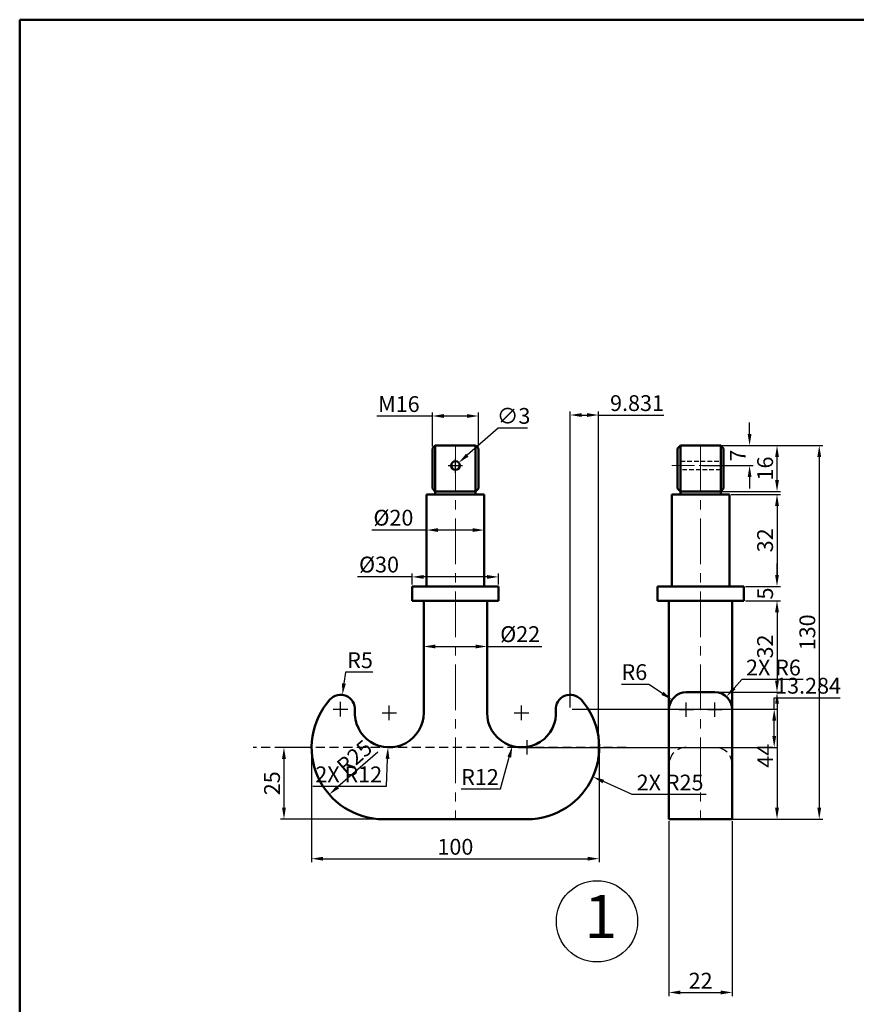
# Model space of a CAD drawing. Units: millimetres. Extents: x -3 to 930, y -425 to 322.
# Tile 3 of 5: x -3 to 288, y -21 to 322. Entities that reach past the tile are written whole.
import ezdxf

# ---------------------------------------------------------------- set-up
doc = ezdxf.new("R2010")
doc.units = ezdxf.units.MM
doc.header["$LTSCALE"] = 0.5
doc.linetypes.add('CENTER', pattern=[50.8, 31.75, -6.35, 6.35, -6.35])
doc.linetypes.add('HIDDEN', pattern=[9.525, 6.35, -3.175])
for name, color, linetype, lineweight in [('M-ANNO-SYMB', 3, 'Continuous', 25), ('M-CNTR', 1, 'CENTER', 18), ('M-DIMS', 2, 'Continuous', 25), ('M-HIDN', 4, 'HIDDEN', 25), ('M-OUTL', 7, 'Continuous', 50), ('M-TEXT', 3, 'Continuous', 25)]:
    doc.layers.add(name, color=color, linetype=linetype, lineweight=lineweight)
doc.styles.get("Standard").update_dxf_attribs({"font": 'arial.ttf'})
doc.dimstyles.new('ISO-25', dxfattribs={"dimtxt": 5.5, "dimasz": 4, "dimexe": 1.25, "dimexo": 0.625, "dimtad": 1, "dimtoh": 1, "dimdec": 0, "dimtxsty": 'Standard', "dimcen": 2.5, "dimadec": 0, "dimazin": 0, "dimtfac": 1, "dimtdec": 0, "dimtofl": 0, "dimtmove": 0, "dimatfit": 3, "dimfxl": 1, "dimarcsym": 0})

# ---------------------------------------------------------------- blocks, each defined once
blk = doc.blocks.new('*D1')
at = {"layer": 'Defpoints', "color": 0, "ltscale": 0.5, "transparency": 16777216}
for p in [(156.9, 183.82), (140.9, 172.56), (156.9, 172.56)]:
    blk.add_point(p, dxfattribs=at)
at = {"layer": 'M-DIMS', "color": 0, "lineweight": -2, "ltscale": 0.5, "transparency": 16777216}
for p, q in [((140.9, 173.18), (140.9, 185.07)), ((156.9, 173.18), (156.9, 185.07)), ((140.9, 183.82), (121.63, 183.82)), ((152.9, 183.82), (144.9, 183.82))]:
    blk.add_line(p, q, dxfattribs=at)
at = {"layer": 'M-DIMS', "color": 0, "ltscale": 0.5, "transparency": 16777216}
for points in [[(144.9, 184.49), (144.9, 183.16), (140.9, 183.82)], [(152.9, 184.49), (152.9, 183.16), (156.9, 183.82)]]:
    blk.add_solid(points, dxfattribs=at)
at = {"layer": 'M-DIMS', "color": 0, "ltscale": 0.5, "transparency": 16777216, "insert": (129.26, 187.26), "char_height": 5.5, "attachment_point": 5}
blk.add_mtext('M16', dxfattribs=at)
blk = doc.blocks.new('*D2')
at = {"layer": 'Defpoints', "color": 0, "ltscale": 0.5, "transparency": 16777216}
for p in [(147.77, 165.57), (150.03, 167.55)]:
    blk.add_point(p, dxfattribs=at)
at = {"layer": 'M-DIMS', "color": 0, "lineweight": -2, "ltscale": 0.5, "transparency": 16777216}
for p, q in [((163.73, 179.55), (153.04, 170.18)), ((173.94, 179.55), (163.73, 179.55)), ((148.9, 164.06), (148.9, 169.06)), ((146.4, 166.56), (151.4, 166.56))]:
    blk.add_line(p, q, dxfattribs=at)
at = {"layer": 'M-DIMS', "color": 0, "ltscale": 0.5, "transparency": 16777216}
blk.add_solid([(152.6, 170.68), (153.48, 169.68), (150.03, 167.55)], dxfattribs=at)
at = {"layer": 'M-DIMS', "color": 0, "ltscale": 0.5, "transparency": 16777216, "insert": (169.15, 183.14), "char_height": 5.5, "attachment_point": 5}
blk.add_mtext('∅3', dxfattribs=at)
blk = doc.blocks.new('*D3')
at = {"layer": 'Defpoints', "color": 0, "ltscale": 0.5, "transparency": 16777216}
for p in [(158.9, 144.14), (138.9, 140.56), (158.9, 140.56)]:
    blk.add_point(p, dxfattribs=at)
at = {"layer": 'M-DIMS', "color": 0, "lineweight": -2, "ltscale": 0.5, "transparency": 16777216}
for p, q in [((138.9, 144.14), (119.81, 144.14)), ((138.9, 141.18), (138.9, 145.39)), ((154.9, 144.14), (142.9, 144.14)), ((158.9, 141.18), (158.9, 145.39))]:
    blk.add_line(p, q, dxfattribs=at)
at = {"layer": 'M-DIMS', "color": 0, "ltscale": 0.5, "transparency": 16777216}
for points in [[(142.9, 144.81), (142.9, 143.48), (138.9, 144.14)], [(154.9, 144.81), (154.9, 143.48), (158.9, 144.14)]]:
    blk.add_solid(points, dxfattribs=at)
at = {"layer": 'M-DIMS', "color": 0, "ltscale": 0.5, "transparency": 16777216, "insert": (127.35, 147.73), "char_height": 5.5, "attachment_point": 5}
blk.add_mtext('%%C20', dxfattribs=at)
blk = doc.blocks.new('*D4')
at = {"layer": 'Defpoints', "color": 0, "ltscale": 0.5, "transparency": 16777216}
for p in [(163.9, 127.84), (133.9, 124.56), (163.9, 124.56)]:
    blk.add_point(p, dxfattribs=at)
at = {"layer": 'M-DIMS', "color": 0, "lineweight": -2, "ltscale": 0.5, "transparency": 16777216}
for p, q in [((133.9, 127.84), (114.81, 127.84)), ((133.9, 125.18), (133.9, 129.09)), ((159.9, 127.84), (137.9, 127.84)), ((163.9, 125.18), (163.9, 129.09))]:
    blk.add_line(p, q, dxfattribs=at)
at = {"layer": 'M-DIMS', "color": 0, "ltscale": 0.5, "transparency": 16777216}
for points in [[(137.9, 128.51), (137.9, 127.18), (133.9, 127.84)], [(159.9, 128.51), (159.9, 127.18), (163.9, 127.84)]]:
    blk.add_solid(points, dxfattribs=at)
at = {"layer": 'M-DIMS', "color": 0, "ltscale": 0.5, "transparency": 16777216, "insert": (122.35, 131.43), "char_height": 5.5, "attachment_point": 5}
blk.add_mtext('%%C30', dxfattribs=at)
blk = doc.blocks.new('*D5')
at = {"layer": 'Defpoints', "color": 0, "ltscale": 0.5, "transparency": 16777216}
for p in [(159.9, 103.64), (137.9, 100.06), (159.9, 100.06)]:
    blk.add_point(p, dxfattribs=at)
at = {"layer": 'M-DIMS', "color": 0, "lineweight": -2, "ltscale": 0.5, "transparency": 16777216}
for p, q in [((137.9, 100.68), (137.9, 104.89)), ((141.9, 103.64), (155.9, 103.64)), ((159.9, 100.68), (159.9, 104.89)), ((159.9, 103.64), (178.96, 103.64))]:
    blk.add_line(p, q, dxfattribs=at)
at = {"layer": 'M-DIMS', "color": 0, "ltscale": 0.5, "transparency": 16777216}
for points in [[(141.9, 104.31), (141.9, 102.98), (137.9, 103.64)], [(155.9, 104.31), (155.9, 102.98), (159.9, 103.64)]]:
    blk.add_solid(points, dxfattribs=at)
at = {"layer": 'M-DIMS', "color": 0, "ltscale": 0.5, "transparency": 16777216, "insert": (171.43, 107.23), "char_height": 5.5, "attachment_point": 5}
blk.add_mtext('%%C22', dxfattribs=at)
blk = doc.blocks.new('*D6')
at = {"layer": 'Defpoints', "color": 0, "ltscale": 0.5, "transparency": 16777216}
for p in [(98.9, 68.56), (89.29, 43.56), (148.9, 43.56)]:
    blk.add_point(p, dxfattribs=at)
at = {"layer": 'M-DIMS', "color": 0, "lineweight": -2, "ltscale": 0.5, "transparency": 16777216}
for p, q in [((98.28, 68.56), (88.04, 68.56)), ((89.29, 64.56), (89.29, 47.56)), ((148.28, 43.56), (88.04, 43.56))]:
    blk.add_line(p, q, dxfattribs=at)
at = {"layer": 'M-DIMS', "color": 0, "ltscale": 0.5, "transparency": 16777216}
for points in [[(88.62, 64.56), (89.95, 64.56), (89.29, 68.56)], [(88.62, 47.56), (89.95, 47.56), (89.29, 43.56)]]:
    blk.add_solid(points, dxfattribs=at)
at = {"layer": 'M-DIMS', "color": 0, "ltscale": 0.5, "transparency": 16777216, "insert": (85.85, 56.06), "char_height": 5.5, "attachment_point": 5, "rotation": 90}
blk.add_mtext('25', dxfattribs=at)
blk = doc.blocks.new('*D7')
at = {"layer": 'Defpoints', "color": 0, "ltscale": 0.5, "transparency": 16777216}
for p in [(98.9, 68.56), (198.9, 68.56), (198.9, 29.83)]:
    blk.add_point(p, dxfattribs=at)
at = {"layer": 'M-DIMS', "color": 0, "lineweight": -2, "ltscale": 0.5, "transparency": 16777216}
for p, q in [((98.9, 67.93), (98.9, 28.58)), ((198.9, 67.93), (198.9, 28.58)), ((102.9, 29.83), (194.9, 29.83))]:
    blk.add_line(p, q, dxfattribs=at)
at = {"layer": 'M-DIMS', "color": 0, "ltscale": 0.5, "transparency": 16777216}
for points in [[(102.9, 30.49), (102.9, 29.16), (98.9, 29.83)], [(194.9, 30.49), (194.9, 29.16), (198.9, 29.83)]]:
    blk.add_solid(points, dxfattribs=at)
at = {"layer": 'M-DIMS', "color": 0, "ltscale": 0.5, "transparency": 16777216, "insert": (148.9, 33.26), "char_height": 5.5, "attachment_point": 5}
blk.add_mtext('100', dxfattribs=at)
blk = doc.blocks.new('*D8')
at = {"layer": 'Defpoints', "color": 0, "ltscale": 0.5, "transparency": 16777216}
for p in [(109.61, 86.8), (108.95, 81.84)]:
    blk.add_point(p, dxfattribs=at)
at = {"layer": 'M-DIMS', "color": 0, "lineweight": -2, "ltscale": 0.5, "transparency": 16777216}
for p, q in [((110.67, 94.73), (110.14, 90.76)), ((120.21, 94.73), (110.67, 94.73)), ((108.95, 79.34), (108.95, 84.34)), ((106.45, 81.84), (111.45, 81.84))]:
    blk.add_line(p, q, dxfattribs=at)
at = {"layer": 'M-DIMS', "color": 0, "ltscale": 0.5, "transparency": 16777216}
blk.add_solid([(109.48, 90.85), (110.8, 90.67), (109.61, 86.8)], dxfattribs=at)
at = {"layer": 'M-DIMS', "color": 0, "ltscale": 0.5, "transparency": 16777216, "insert": (115.75, 98.15), "char_height": 5.5, "attachment_point": 5}
blk.add_mtext('R5', dxfattribs=at)
blk = doc.blocks.new('*D9')
at = {"layer": 'Defpoints', "color": 0, "ltscale": 0.5, "transparency": 16777216}
for p in [(171.9, 80.56), (168.71, 68.99)]:
    blk.add_point(p, dxfattribs=at)
at = {"layer": 'M-DIMS', "color": 0, "lineweight": -2, "ltscale": 0.5, "transparency": 16777216}
for p, q in [((171.9, 78.06), (171.9, 83.06)), ((169.4, 80.56), (174.4, 80.56)), ((164.62, 54.15), (167.65, 65.13)), ((150.91, 54.15), (164.62, 54.15))]:
    blk.add_line(p, q, dxfattribs=at)
at = {"layer": 'M-DIMS', "color": 0, "ltscale": 0.5, "transparency": 16777216}
blk.add_solid([(167, 65.31), (168.29, 64.96), (168.71, 68.99)], dxfattribs=at)
at = {"layer": 'M-DIMS', "color": 0, "ltscale": 0.5, "transparency": 16777216, "insert": (157.45, 57.53), "char_height": 5.5, "attachment_point": 5}
blk.add_mtext('R12', dxfattribs=at)
blk = doc.blocks.new('*D10')
at = {"layer": 'Defpoints', "color": 0, "ltscale": 0.5, "transparency": 16777216}
for p in [(123.9, 68.56), (105.03, 52.17)]:
    blk.add_point(p, dxfattribs=at)
at = {"layer": 'M-DIMS', "color": 0, "lineweight": -2, "ltscale": 0.5, "transparency": 16777216}
blk.add_line((121.96, 66.87), (108.05, 54.79), dxfattribs=at)
at = {"layer": 'M-DIMS', "color": 0, "ltscale": 0.5, "transparency": 16777216}
blk.add_solid([(107.61, 55.29), (108.48, 54.29), (105.03, 52.17)], dxfattribs=at)
at = {"layer": 'M-DIMS', "color": 0, "ltscale": 0.5, "transparency": 16777216, "insert": (114.26, 64.74), "char_height": 5.5, "attachment_point": 5, "rotation": 40.9701}
blk.add_mtext('R25', dxfattribs=at)
blk = doc.blocks.new('*D11')
at = {"layer": 'Defpoints', "color": 0, "ltscale": 0.5, "transparency": 16777216}
for p in [(224.23, 85.1), (229.18, 81.71)]:
    blk.add_point(p, dxfattribs=at)
at = {"layer": 'M-DIMS', "color": 0, "lineweight": -2, "ltscale": 0.5, "transparency": 16777216}
for p, q in [((206.71, 90.58), (216.2, 90.58)), ((216.2, 90.58), (220.93, 87.36)), ((229.18, 79.21), (229.18, 84.21)), ((226.68, 81.71), (231.68, 81.71))]:
    blk.add_line(p, q, dxfattribs=at)
at = {"layer": 'M-DIMS', "color": 0, "ltscale": 0.5, "transparency": 16777216}
blk.add_solid([(221.3, 87.91), (220.55, 86.81), (224.23, 85.1)], dxfattribs=at)
at = {"layer": 'M-DIMS', "color": 0, "ltscale": 0.5, "transparency": 16777216, "insert": (211.15, 94.02), "char_height": 5.5, "attachment_point": 5}
blk.add_mtext('R6', dxfattribs=at)
blk = doc.blocks.new('*D12')
at = {"layer": 'Defpoints', "color": 0, "ltscale": 0.5, "transparency": 16777216}
for p in [(234.18, 173.56), (234.18, 166.56), (251.21, 166.56)]:
    blk.add_point(p, dxfattribs=at)
at = {"layer": 'M-DIMS', "color": 0, "lineweight": -2, "ltscale": 0.5, "transparency": 16777216}
for p, q in [((251.21, 177.56), (251.21, 181.56)), ((234.81, 173.56), (252.46, 173.56)), ((234.81, 166.56), (252.46, 166.56)), ((251.21, 162.56), (251.21, 158.56))]:
    blk.add_line(p, q, dxfattribs=at)
at = {"layer": 'M-DIMS', "color": 0, "ltscale": 0.5, "transparency": 16777216}
for points in [[(250.55, 177.56), (251.88, 177.56), (251.21, 173.56)], [(250.55, 162.56), (251.88, 162.56), (251.21, 166.56)]]:
    blk.add_solid(points, dxfattribs=at)
at = {"layer": 'M-DIMS', "color": 0, "ltscale": 0.5, "transparency": 16777216, "insert": (247.84, 170.06), "char_height": 5.5, "attachment_point": 5, "rotation": 90}
blk.add_mtext('7', dxfattribs=at)
blk = doc.blocks.new('*D13')
at = {"layer": 'Defpoints', "color": 0, "ltscale": 0.5, "transparency": 16777216}
for p in [(243.63, 173.56), (260.75, 173.56), (234.18, 157.56)]:
    blk.add_point(p, dxfattribs=at)
at = {"layer": 'M-DIMS', "color": 0, "lineweight": -2, "ltscale": 0.5, "transparency": 16777216}
for p, q in [((244.26, 173.56), (262, 173.56)), ((260.75, 161.56), (260.75, 169.56)), ((234.81, 157.56), (262, 157.56))]:
    blk.add_line(p, q, dxfattribs=at)
at = {"layer": 'M-DIMS', "color": 0, "ltscale": 0.5, "transparency": 16777216}
for points in [[(260.08, 169.56), (261.42, 169.56), (260.75, 173.56)], [(260.08, 161.56), (261.42, 161.56), (260.75, 157.56)]]:
    blk.add_solid(points, dxfattribs=at)
at = {"layer": 'M-DIMS', "color": 0, "ltscale": 0.5, "transparency": 16777216, "insert": (257.32, 165.56), "char_height": 5.5, "attachment_point": 5, "rotation": 90}
blk.add_mtext('16', dxfattribs=at)
blk = doc.blocks.new('*D14')
at = {"layer": 'Defpoints', "color": 0, "ltscale": 0.5, "transparency": 16777216}
for p in [(244.18, 156.56), (249.18, 124.56), (260.75, 124.56)]:
    blk.add_point(p, dxfattribs=at)
at = {"layer": 'M-DIMS', "color": 0, "lineweight": -2, "ltscale": 0.5, "transparency": 16777216}
for p, q in [((244.81, 156.56), (262, 156.56)), ((260.75, 152.56), (260.75, 128.56)), ((249.81, 124.56), (262, 124.56))]:
    blk.add_line(p, q, dxfattribs=at)
at = {"layer": 'M-DIMS', "color": 0, "ltscale": 0.5, "transparency": 16777216}
for points in [[(260.08, 152.56), (261.42, 152.56), (260.75, 156.56)], [(260.08, 128.56), (261.42, 128.56), (260.75, 124.56)]]:
    blk.add_solid(points, dxfattribs=at)
at = {"layer": 'M-DIMS', "color": 0, "ltscale": 0.5, "transparency": 16777216, "insert": (257.31, 140.56), "char_height": 5.5, "attachment_point": 5, "rotation": 90}
blk.add_mtext('32', dxfattribs=at)
blk = doc.blocks.new('*D15')
at = {"layer": 'Defpoints', "color": 0, "ltscale": 0.5, "transparency": 16777216}
for p in [(249.18, 124.56), (249.18, 119.56), (260.75, 119.56)]:
    blk.add_point(p, dxfattribs=at)
at = {"layer": 'M-DIMS', "color": 0, "lineweight": -2, "ltscale": 0.5, "transparency": 16777216}
for p, q in [((260.75, 128.56), (260.75, 132.56)), ((249.81, 124.56), (262, 124.56)), ((249.81, 119.56), (262, 119.56)), ((260.75, 115.56), (260.75, 111.56))]:
    blk.add_line(p, q, dxfattribs=at)
at = {"layer": 'M-DIMS', "color": 0, "ltscale": 0.5, "transparency": 16777216}
for points in [[(260.08, 128.56), (261.42, 128.56), (260.75, 124.56)], [(260.08, 115.56), (261.42, 115.56), (260.75, 119.56)]]:
    blk.add_solid(points, dxfattribs=at)
at = {"layer": 'M-DIMS', "color": 0, "ltscale": 0.5, "transparency": 16777216, "insert": (257.33, 122.06), "char_height": 5.5, "attachment_point": 5, "rotation": 90}
blk.add_mtext('5', dxfattribs=at)
blk = doc.blocks.new('*D16')
at = {"layer": 'Defpoints', "color": 0, "ltscale": 0.5, "transparency": 16777216}
for p in [(249.18, 119.56), (234.18, 87.71), (260.75, 87.71)]:
    blk.add_point(p, dxfattribs=at)
at = {"layer": 'M-DIMS', "color": 0, "lineweight": -2, "ltscale": 0.5, "transparency": 16777216}
for p, q in [((249.81, 119.56), (262, 119.56)), ((260.75, 115.56), (260.75, 91.71)), ((234.81, 87.71), (262, 87.71))]:
    blk.add_line(p, q, dxfattribs=at)
at = {"layer": 'M-DIMS', "color": 0, "ltscale": 0.5, "transparency": 16777216}
for points in [[(260.08, 115.56), (261.42, 115.56), (260.75, 119.56)], [(260.08, 91.71), (261.42, 91.71), (260.75, 87.71)]]:
    blk.add_solid(points, dxfattribs=at)
at = {"layer": 'M-DIMS', "color": 0, "ltscale": 0.5, "transparency": 16777216, "insert": (257.31, 103.64), "char_height": 5.5, "attachment_point": 5, "rotation": 90}
blk.add_mtext('32', dxfattribs=at)
blk = doc.blocks.new('*D17')
at = {"layer": 'Defpoints', "color": 0, "ltscale": 0.5, "transparency": 16777216}
for p in [(234.18, 173.56), (234.18, 43.56), (275.44, 43.56)]:
    blk.add_point(p, dxfattribs=at)
at = {"layer": 'M-DIMS', "color": 0, "lineweight": -2, "ltscale": 0.5, "transparency": 16777216}
for p, q in [((234.81, 173.56), (276.69, 173.56)), ((275.44, 169.56), (275.44, 47.56)), ((234.81, 43.56), (276.69, 43.56))]:
    blk.add_line(p, q, dxfattribs=at)
at = {"layer": 'M-DIMS', "color": 0, "ltscale": 0.5, "transparency": 16777216}
for points in [[(274.78, 169.56), (276.11, 169.56), (275.44, 173.56)], [(274.78, 47.56), (276.11, 47.56), (275.44, 43.56)]]:
    blk.add_solid(points, dxfattribs=at)
at = {"layer": 'M-DIMS', "color": 0, "ltscale": 0.5, "transparency": 16777216, "insert": (272.01, 108.56), "char_height": 5.5, "attachment_point": 5, "rotation": 90}
blk.add_mtext('130', dxfattribs=at)
blk = doc.blocks.new('*D18')
at = {"layer": 'Defpoints', "color": 0, "ltscale": 0.5, "transparency": 16777216}
for p in [(234.18, 87.71), (234.18, 43.56), (260.75, 43.56)]:
    blk.add_point(p, dxfattribs=at)
at = {"layer": 'M-DIMS', "color": 0, "lineweight": -2, "ltscale": 0.5, "transparency": 16777216}
for p, q in [((234.81, 87.71), (262, 87.71)), ((260.75, 83.71), (260.75, 47.56)), ((234.81, 43.56), (262, 43.56))]:
    blk.add_line(p, q, dxfattribs=at)
at = {"layer": 'M-DIMS', "color": 0, "ltscale": 0.5, "transparency": 16777216}
for points in [[(260.08, 83.71), (261.42, 83.71), (260.75, 87.71)], [(260.08, 47.56), (261.42, 47.56), (260.75, 43.56)]]:
    blk.add_solid(points, dxfattribs=at)
at = {"layer": 'M-DIMS', "color": 0, "ltscale": 0.5, "transparency": 16777216, "insert": (257.37, 65.64), "char_height": 5.5, "attachment_point": 5, "rotation": 90}
blk.add_mtext('44', dxfattribs=at)
blk = doc.blocks.new('BALLOON')
at = {"ltscale": 0.5}
blk.add_circle((198.15, 8.03), 14.13, dxfattribs=at)
blk = doc.blocks.new('*D83')
at = {"layer": 'Defpoints', "color": 0, "ltscale": 0.5, "transparency": 16777216}
for p in [(198.68, 184.16), (188.85, 81.84), (198.68, 65.26)]:
    blk.add_point(p, dxfattribs=at)
at = {"layer": 'M-DIMS', "color": 0, "lineweight": -2, "ltscale": 0.5, "transparency": 16777216}
for p, q in [((188.85, 82.47), (188.85, 185.41)), ((198.68, 65.89), (198.68, 185.41)), ((192.85, 184.16), (194.68, 184.16)), ((198.68, 184.16), (221.43, 184.16))]:
    blk.add_line(p, q, dxfattribs=at)
at = {"layer": 'M-DIMS', "color": 0, "ltscale": 0.5, "transparency": 16777216}
for points in [[(192.85, 184.82), (192.85, 183.49), (188.85, 184.16)], [(194.68, 184.82), (194.68, 183.49), (198.68, 184.16)]]:
    blk.add_solid(points, dxfattribs=at)
at = {"layer": 'M-DIMS', "color": 0, "ltscale": 0.5, "transparency": 16777216, "insert": (212.06, 187.59), "char_height": 5.5, "attachment_point": 5}
blk.add_mtext('9.831', dxfattribs=at)
blk = doc.blocks.new('*D84')
at = {"layer": 'Defpoints', "color": 0, "ltscale": 0.5, "transparency": 16777216}
for p in [(188.85, 81.84), (259.78, 81.84), (173.9, 68.56)]:
    blk.add_point(p, dxfattribs=at)
at = {"layer": 'M-DIMS', "color": 0, "lineweight": -2, "ltscale": 0.5, "transparency": 16777216}
for p, q in [((259.78, 81.84), (259.78, 85.84)), ((259.78, 85.84), (282.7, 85.84)), ((189.48, 81.84), (261.03, 81.84)), ((259.78, 72.56), (259.78, 77.84)), ((174.53, 68.56), (261.03, 68.56))]:
    blk.add_line(p, q, dxfattribs=at)
at = {"layer": 'M-DIMS', "color": 0, "ltscale": 0.5, "transparency": 16777216}
for points in [[(259.11, 77.84), (260.45, 77.84), (259.78, 81.84)], [(259.11, 72.56), (260.45, 72.56), (259.78, 68.56)]]:
    blk.add_solid(points, dxfattribs=at)
at = {"layer": 'M-DIMS', "color": 0, "ltscale": 0.5, "transparency": 16777216, "insert": (271.55, 89.28), "char_height": 5.5, "attachment_point": 5}
blk.add_mtext('13.284', dxfattribs=at)
blk = doc.blocks.new('*D85')
at = {"layer": 'Defpoints', "color": 0, "ltscale": 0.5, "transparency": 16777216}
for p in [(223.18, 43.56), (245.18, 43.56), (245.18, -16.7)]:
    blk.add_point(p, dxfattribs=at)
at = {"layer": 'M-DIMS', "color": 0, "lineweight": -2, "ltscale": 0.5, "transparency": 16777216}
for p, q in [((223.18, 42.93), (223.18, -17.95)), ((245.18, 42.93), (245.18, -17.95)), ((227.18, -16.7), (241.18, -16.7))]:
    blk.add_line(p, q, dxfattribs=at)
at = {"layer": 'M-DIMS', "color": 0, "ltscale": 0.5, "transparency": 16777216}
for points in [[(227.18, -16.03), (227.18, -17.37), (223.18, -16.7)], [(241.18, -16.03), (241.18, -17.37), (245.18, -16.7)]]:
    blk.add_solid(points, dxfattribs=at)
at = {"layer": 'M-DIMS', "color": 0, "ltscale": 0.5, "transparency": 16777216, "insert": (234.18, -13.31), "char_height": 5.5, "attachment_point": 5}
blk.add_mtext('22', dxfattribs=at)
blk = doc.blocks.new('*D89')
at = {"layer": 'Defpoints', "color": 0, "ltscale": 0.5, "transparency": 16777216}
for p in [(173.9, 68.56), (196.71, 58.31)]:
    blk.add_point(p, dxfattribs=at)
at = {"layer": 'M-DIMS', "color": 0, "lineweight": -2, "ltscale": 0.5, "transparency": 16777216}
for p, q in [((171.4, 68.56), (176.4, 68.56)), ((173.9, 66.06), (173.9, 71.06)), ((210.39, 52.17), (200.36, 56.67)), ((236.11, 52.17), (210.39, 52.17))]:
    blk.add_line(p, q, dxfattribs=at)
at = {"layer": 'M-DIMS', "color": 0, "ltscale": 0.5, "transparency": 16777216}
blk.add_solid([(200.63, 57.28), (200.08, 56.07), (196.71, 58.31)], dxfattribs=at)
at = {"layer": 'M-DIMS', "color": 0, "ltscale": 0.5, "transparency": 16777216, "insert": (223.56, 55.6), "char_height": 5.5, "attachment_point": 5}
blk.add_mtext('2X R25', dxfattribs=at)
blk = doc.blocks.new('*D90')
at = {"layer": 'Defpoints', "color": 0, "ltscale": 0.5, "transparency": 16777216}
for p in [(125.9, 80.56), (125.45, 68.57)]:
    blk.add_point(p, dxfattribs=at)
at = {"layer": 'M-DIMS', "color": 0, "lineweight": -2, "ltscale": 0.5, "transparency": 16777216}
for p, q in [((125.9, 78.06), (125.9, 83.06)), ((123.4, 80.56), (128.4, 80.56)), ((124.94, 55.05), (125.3, 64.57)), ((99.32, 55.05), (124.94, 55.05))]:
    blk.add_line(p, q, dxfattribs=at)
at = {"layer": 'M-DIMS', "color": 0, "ltscale": 0.5, "transparency": 16777216}
blk.add_solid([(124.63, 64.59), (125.96, 64.54), (125.45, 68.57)], dxfattribs=at)
at = {"layer": 'M-DIMS', "color": 0, "ltscale": 0.5, "transparency": 16777216, "insert": (111.81, 58.44), "char_height": 5.5, "attachment_point": 5}
blk.add_mtext('2X R12', dxfattribs=at)
blk = doc.blocks.new('*D91')
at = {"layer": 'Defpoints', "color": 0, "ltscale": 0.5, "transparency": 16777216}
for p in [(243.17, 86.19), (239.18, 81.71)]:
    blk.add_point(p, dxfattribs=at)
at = {"layer": 'M-DIMS', "color": 0, "lineweight": -2, "ltscale": 0.5, "transparency": 16777216}
for p, q in [((248.49, 92.17), (245.83, 89.18)), ((269.9, 92.17), (248.49, 92.17)), ((239.18, 79.21), (239.18, 84.21)), ((236.68, 81.71), (241.68, 81.71))]:
    blk.add_line(p, q, dxfattribs=at)
at = {"layer": 'M-DIMS', "color": 0, "ltscale": 0.5, "transparency": 16777216}
blk.add_solid([(245.34, 89.62), (246.33, 88.74), (243.17, 86.19)], dxfattribs=at)
at = {"layer": 'M-DIMS', "color": 0, "ltscale": 0.5, "transparency": 16777216, "insert": (259.51, 95.6), "char_height": 5.5, "attachment_point": 5}
blk.add_mtext('2X R6', dxfattribs=at)

msp = doc.modelspace()

# ---------------------------------------------------------------- linework, layer by layer
at = {"layer": 'M-CNTR'}
for p, q in [((148.9019, 173.5576), (148.9019, 43.5576)), ((234.1804, 173.5576), (234.1804, 43.5576))]:
    msp.add_line(p, q, dxfattribs=at)
at = {"layer": 'M-CNTR', "ltscale": 0.5}
msp.add_line((224.1276, 166.5576), (247.1768, 166.5576), dxfattribs=at)
at = {"layer": 'M-HIDN'}
msp.add_line((208.3227, 68.5576), (78.5676, 68.5576), dxfattribs=at)
at = {"layer": 'M-HIDN', "ltscale": 0.5}
msp.add_line((229.1804, 68.5576), (239.1804, 68.5576), dxfattribs=at)
for points in [[(227.1804, 168.0576), (234.1804, 168.0576), (241.1804, 168.0576)], [(241.1804, 165.0576), (234.1804, 165.0576), (227.1804, 165.0576)]]:
    msp.add_lwpolyline(points, dxfattribs=at)
at = {"layer": 'M-HIDN'}
for centre, start, end in [((229.1804, 62.5576), 90, 180), ((239.1804, 62.5576), 360, 90)]:
    msp.add_arc(centre, 6, start, end, dxfattribs=at)
at = {"layer": 'M-OUTL'}
for p, q in [((140.9019, 172.5576), (141.9019, 173.5576)), ((140.9019, 158.5576), (140.9019, 172.5576)), ((141.9019, 173.5576), (155.9019, 173.5576)), ((141.9019, 173.5576), (141.9019, 156.5576)), ((156.9019, 172.5576), (155.9019, 173.5576)), ((155.9019, 173.5576), (155.9019, 156.5576)), ((156.9019, 172.5576), (156.9019, 158.5576)), ((226.1804, 172.5576), (227.1804, 173.5576)), ((226.1804, 158.5576), (226.1804, 172.5576)), ((227.1804, 173.5576), (241.1804, 173.5576)), ((227.1804, 173.5576), (227.1804, 156.5576)), ((242.1804, 172.5576), (241.1804, 173.5576)), ((241.1804, 173.5576), (241.1804, 156.5576)), ((242.1804, 172.5576), (242.1804, 158.5576)), ((140.9019, 158.5576), (141.9019, 157.5576)), ((155.9019, 157.5576), (141.9019, 157.5576)), ((156.9019, 158.5576), (155.9019, 157.5576)), ((226.1804, 158.5576), (227.1804, 157.5576)), ((241.1804, 157.5576), (227.1804, 157.5576)), ((242.1804, 158.5576), (241.1804, 157.5576)), ((138.9019, 156.5576), (158.9019, 156.5576)), ((138.9019, 124.5576), (138.9019, 156.5576)), ((155.9019, 156.5576), (141.9019, 156.5576)), ((158.9019, 156.5576), (158.9019, 124.5576)), ((224.1804, 156.5576), (244.1804, 156.5576)), ((224.1804, 124.5576), (224.1804, 156.5576)), ((241.1804, 156.5576), (227.1804, 156.5576)), ((244.1804, 156.5576), (244.1804, 124.5576)), ((133.9019, 119.5576), (133.9019, 124.5576)), ((133.9019, 124.5576), (158.9019, 124.5576)), ((158.9019, 124.5576), (138.9019, 124.5576)), ((158.9019, 124.5576), (163.9019, 124.5576)), ((163.9019, 124.5576), (163.9019, 119.5576)), ((219.1804, 119.5576), (219.1804, 124.5576)), ((219.1804, 124.5576), (244.1804, 124.5576)), ((244.1804, 124.5576), (224.1804, 124.5576)), ((244.1804, 124.5576), (249.1804, 124.5576)), ((249.1804, 124.5576), (249.1804, 119.5576)), ((163.9019, 119.5576), (133.9019, 119.5576)), ((137.9019, 119.5576), (137.9019, 80.5576)), ((159.9019, 119.5576), (159.9019, 80.5576)), ((249.1804, 119.5576), (219.1804, 119.5576)), ((223.1804, 119.5576), (223.1804, 43.5576)), ((245.1804, 119.5576), (245.1804, 43.5576)), ((173.9019, 43.5576), (123.9019, 43.5576))]:
    msp.add_line(p, q, dxfattribs=at)
at = {"layer": 'M-OUTL', "ltscale": 0.5}
for p, q in [((229.1804, 87.713), (239.1804, 87.713)), ((223.1804, 43.5576), (245.1804, 43.5576))]:
    msp.add_line(p, q, dxfattribs=at)
msp.add_lwpolyline([(-2.6134, 321.6785), (929.6113, 321.6785), (929.6113, -424.8872), (-2.6134, -424.8872)], close=True, dxfattribs=at)
msp.add_circle((148.9019, 166.5576), 1.5, dxfattribs=at)
at = {"layer": 'M-OUTL'}
for centre, radius, start, end in [((108.9504, 81.8412), 5, 355.669782, 138.380633), ((188.8533, 81.8412), 5, 41.619367, 184.330218), ((229.1804, 81.713), 6, 90, 180), ((239.1804, 81.713), 6, 360, 90), ((123.9019, 68.5576), 25, 138.380633, 270), ((173.9019, 68.5576), 25, 270, 41.619367), ((125.9019, 80.5576), 12, 175.669782, 0), ((171.9019, 80.5576), 12, 180, 4.330218)]:
    msp.add_arc(centre, radius, start, end, dxfattribs=at)

# ---------------------------------------------------------------- block references
at = {"layer": 'M-ANNO-SYMB'}
msp.add_blockref('BALLOON', (0, 0), dxfattribs=at)

# ---------------------------------------------------------------- texts
at = {"layer": 'M-TEXT', "ltscale": 0.5, "insert": (193.7518, 17.2084), "char_height": 15, "attachment_point": 1}
msp.add_mtext_dynamic_manual_height_columns('1', width=15, gutter_width=12.5, heights=[0], dxfattribs=at)

# ---------------------------------------------------------------- dimensions: what is measured, and where the dimension line sits
at = {"layer": 'M-DIMS', "ltscale": 0.5}
for base, p1, p2, text, picture, middle in [((156.9019, 183.8226), (140.9019, 172.5576), (156.9019, 172.5576), 'M<>', '*D1', (129.2649, 183.8226)), ((158.9019, 144.1446), (138.9019, 140.5576), (158.9019, 140.5576), '%%C<>', '*D3', (127.355, 144.1446)), ((163.9019, 127.8438), (133.9019, 124.5576), (163.9019, 124.5576), '%%C<>', '*D4', (122.355, 127.8438)), ((159.9019, 103.6446), (137.9019, 100.0576), (159.9019, 100.0576), '%%C<>', '*D5', (171.43, 103.6446))]:
    dim = msp.add_linear_dim(base=base, p1=p1, p2=p2, text=text, dimstyle='ISO-25', override={"dimclrd": 0, "dimclre": 0, "dimclrt": 0}, dxfattribs=at)
    dim.commit()
    dim.dimension.update_dxf_attribs({"geometry": picture, "text_midpoint": middle, "dimtype": 160})
for base, p1, p2, override, picture, middle in [((198.6847, 184.1576), (188.8533, 81.8412), (198.6847, 65.2618), {"dimdec": 3, "dimlfac": 1, "dimrnd": 0, "dimzin": 0, "dimdsep": 46, "dimlunit": 2}, '*D83', (212.0586, 187.5926)), ((198.9019, 29.8262), (98.9019, 68.5576), (198.9019, 68.5576), {"dimclrd": 0, "dimclre": 0, "dimclrt": 0}, '*D7', (148.9019, 33.2594)), ((245.1804, -16.6995), (223.1804, 43.5576), (245.1804, 43.5576), {"dimdec": 0, "dimlfac": 1, "dimrnd": 0, "dimzin": 0, "dimdsep": 46, "dimlunit": 2}, '*D85', (234.1804, -13.3132))]:
    dim = msp.add_linear_dim(base=base, p1=p1, p2=p2, dimstyle='ISO-25', override=override, dxfattribs=at)
    dim.commit()
    dim.dimension.update_dxf_attribs({"geometry": picture, "text_midpoint": middle})
dim = msp.add_diameter_dim_2p(p1=(147.7738, 165.5689), p2=(150.0299, 167.5463), dimstyle='ISO-25', override={"dimclrd": 0, "dimclre": 0, "dimclrt": 0}, dxfattribs=at)
dim.commit()
dim.dimension.update_dxf_attribs({"geometry": '*D2', "text_midpoint": (169.1455, 179.551), "dimtype": 163})
for base, p1, p2, override, picture, middle in [((251.2118, 166.5576), (234.1804, 173.5576), (234.1804, 166.5576), {"dimclrd": 0, "dimclre": 0, "dimclrt": 0}, '*D12', (247.8368, 170.0576)), ((260.7486, 173.5576), (234.1804, 157.5576), (243.6336, 173.5576), {"dimclrd": 0, "dimclre": 0, "dimclrt": 0}, '*D13', (257.3154, 165.5576)), ((275.4449, 43.5576), (234.1804, 173.5576), (234.1804, 43.5576), {"dimclrd": 0, "dimclre": 0, "dimclrt": 0}, '*D17', (272.0099, 108.5576)), ((260.7486, 124.5576), (244.1804, 156.5576), (249.1804, 124.5576), {"dimclrd": 0, "dimclre": 0, "dimclrt": 0}, '*D14', (257.3136, 140.5576)), ((260.7486, 119.5576), (249.1804, 124.5576), (249.1804, 119.5576), {"dimclrd": 0, "dimclre": 0, "dimclrt": 0}, '*D15', (257.3267, 122.0576)), ((260.7486, 87.713), (249.1804, 119.5576), (234.1804, 87.713), {"dimclrd": 0, "dimclre": 0, "dimclrt": 0}, '*D16', (257.3136, 103.6353)), ((259.7804, 81.8412), (173.9019, 68.5576), (188.8533, 81.8412), {"dimdec": 3, "dimlfac": 1, "dimrnd": 0, "dimzin": 0, "dimdsep": 46, "dimlunit": 2}, '*D84', (271.5518, 89.2762)), ((260.7486, 43.5576), (234.1804, 87.713), (234.1804, 43.5576), {"dimclrd": 0, "dimclre": 0, "dimclrt": 0}, '*D18', (257.3736, 65.6353)), ((89.2868, 43.5576), (98.9019, 68.5576), (148.9019, 43.5576), {"dimclrd": 0, "dimclre": 0, "dimclrt": 0}, '*D6', (85.8536, 56.0576))]:
    dim = msp.add_linear_dim(base=base, p1=p1, p2=p2, angle=90, dimstyle='ISO-25', override=override, dxfattribs=at)
    dim.commit()
    dim.dimension.update_dxf_attribs({"geometry": picture, "text_midpoint": middle})
for center, mpoint, picture, middle in [((239.1804, 81.713), (243.1718, 86.1929), '*D91', (259.5072, 95.5991)), ((125.9019, 80.5576), (125.449, 68.5662), '*D90', (111.8147, 58.4377))]:
    dim = msp.add_radius_dim(center=center, mpoint=mpoint, text='2X <>', dimstyle='ISO-25', override={"dimdec": 0, "dimlfac": 1, "dimrnd": 0, "dimzin": 0, "dimdsep": 46, "dimlunit": 2}, dxfattribs=at)
    dim.commit()
    dim.dimension.update_dxf_attribs({"geometry": picture, "text_midpoint": middle})
dim = msp.add_radius_dim(center=(108.9504, 81.8412), mpoint=(109.6131, 86.7971), dimstyle='ISO-25', override={"dimclrd": 0, "dimclre": 0, "dimclrt": 0}, dxfattribs=at)
dim.commit()
dim.dimension.update_dxf_attribs({"geometry": '*D8', "text_midpoint": (115.7535, 98.1484)})
for center, mpoint, picture, middle in [((229.1804, 81.713), (224.2272, 85.0992), '*D11', (211.146, 90.5843)), ((171.9019, 80.5576), (168.7107, 68.9897), '*D9', (157.448, 54.1466)), ((123.9019, 68.5576), (105.0256, 52.166), '*D10', (116.515, 62.1431))]:
    dim = msp.add_radius_dim(center=center, mpoint=mpoint, dimstyle='ISO-25', override={"dimclrd": 0, "dimclre": 0, "dimclrt": 0}, dxfattribs=at)
    dim.commit()
    dim.dimension.update_dxf_attribs({"geometry": picture, "text_midpoint": middle, "dimtype": 164})
dim = msp.add_radius_dim(center=(173.9019, 68.5576), mpoint=(196.7065, 58.3132), text='2X <>', dimstyle='ISO-25', override={"dimdec": 0, "dimlfac": 1, "dimrnd": 0, "dimzin": 0, "dimdsep": 46, "dimlunit": 2}, dxfattribs=at)
dim.commit()
dim.dimension.update_dxf_attribs({"geometry": '*D89', "text_midpoint": (223.5619, 52.1666), "dimtype": 164})

doc.saveas('drawing.dxf')
